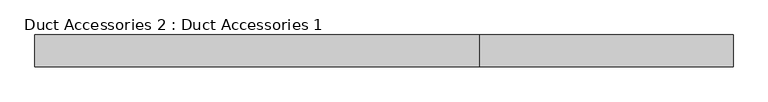
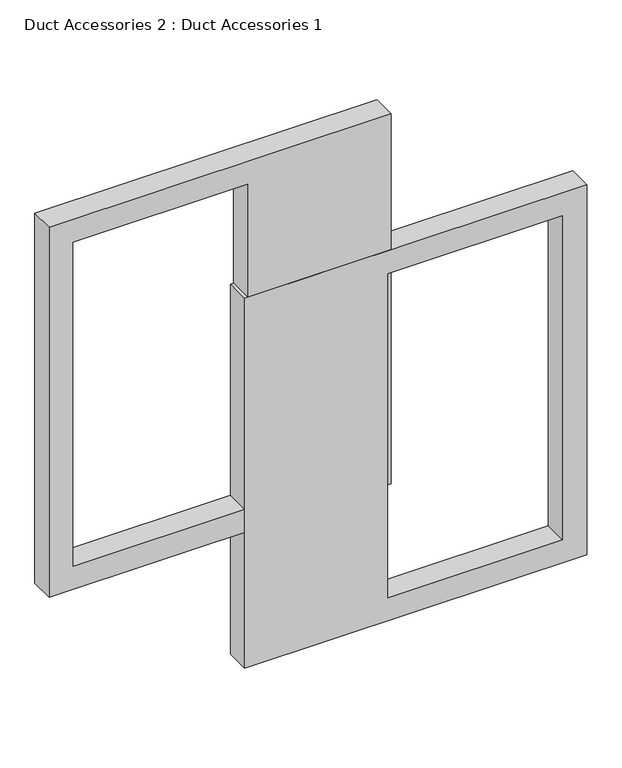
"""IFC4 building model written with IfcOpenShell, lengths in millimetres: damper geometry, Duct Accessories 2 : Duct Accessories 1."""

from ifc_helpers import new_model, si_unit, frame, origin, place, context, project, spatial, polyline, outline, extrude, source, transform, mapped, element, save


def duct_accessories_2_duct_accessories_1_b7e40825(model_context):
    return source(origin(), model_context, "Body", "SweptSolid", [
        extrude(outline(polyline([(35327.1403114, -12928.36893), (34107.9403114, -12928.36893), (34107.9403114, -11861.56893), (35327.1403114, -11861.56893), (35327.1403114, -12928.36893)]), holes=[polyline([(35250.9403114, -12480.9324751), (35250.9403114, -11937.76893), (34184.1403114, -11937.76893), (34184.1403114, -12480.9324751), (35250.9403114, -12480.9324751)])]), frame((0.0, -447.4934478, 0.0), z_axis=(0.0, 1.0, 0.0), x_axis=(0.0, 0.0, 1.0)), (0.0, 0.0, 1.0), 76.2),
        extrude(outline(polyline([(35774.5767663, -12471.5606701), (35774.5767663, -13538.3606701), (34555.3767663, -13538.3606701), (34555.3767663, -12471.5606701), (35774.5767663, -12471.5606701)]), holes=[polyline([(35698.3767663, -12918.997125), (34631.5767663, -12918.997125), (34631.5767663, -13462.1606701), (35698.3767663, -13462.1606701), (35698.3767663, -12918.997125)])]), frame((0.0, -447.4934478, 0.0), z_axis=(0.0, 1.0, 0.0), x_axis=(0.0, 0.0, 1.0)), (0.0, 0.0, 1.0), 76.2),
    ])


if __name__ == "__main__":
    model = new_model("IFC4")
    model_context = context("Model", 3, world=origin())
    ifc_project = project(units=[si_unit("LENGTHUNIT", "METRE", prefix="MILLI")], contexts=[model_context])
    site = spatial("IfcSite", under=ifc_project)
    building = spatial("IfcBuilding", under=site)
    placement = place(None, origin())
    duct_accessories_2_duct_accessories_1_shape = duct_accessories_2_duct_accessories_1_b7e40825(model_context)
    element("IfcDamper", 1, ObjectType="Duct Accessories 2 : Duct Accessories 1", at=placement, inside=building, context=model_context, shape_type="MappedRepresentation", body=[
        mapped(duct_accessories_2_duct_accessories_1_shape, transform((0.0, 0.0, 0.0), x_axis=(1.0, 0.0, 0.0), y_axis=(0.0, 1.0, 0.0), z_axis=(0.0, 0.0, 1.0))),
    ])
    save(model, "model.ifc")

# Revit data of these elements
# Element 1 (IfcDamper, "Duct Accessories 2 : Duct Accessories 1")
#   Materials on its faces: "border"
# Materials
#   "border": class "Generic", colour RGB 144 144 144, transparency 0, Cost = 0
